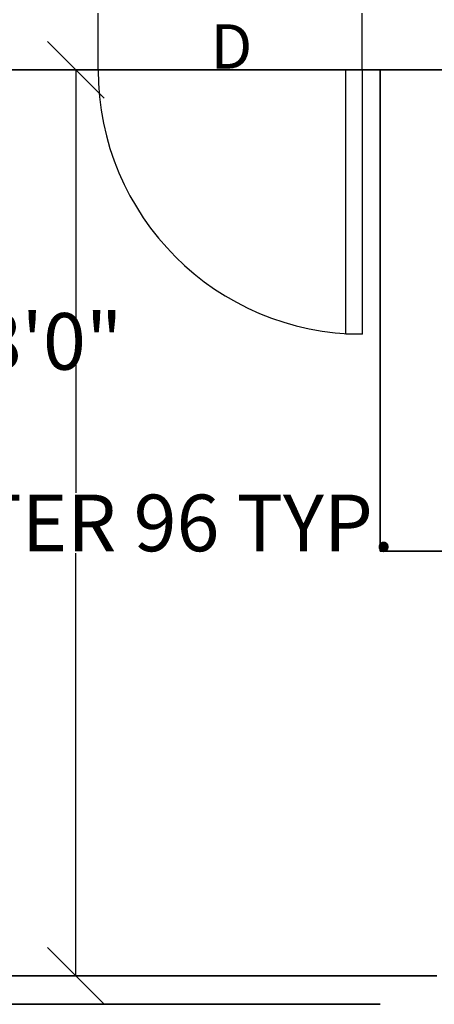
# Model space of a CAD drawing. Units: inches. Extents: x -1198 to -69, y -512 to 437.
# Tile 41 of 50: x -610 to -566, y 158 to 263. Entities that reach past the tile are written whole.
import ezdxf

# ---------------------------------------------------------------- set-up
doc = ezdxf.new("R2010")
doc.units = ezdxf.units.IN
doc.header["$MEASUREMENT"] = 0
for name, color, linetype, lineweight in [('A-ANNO-DIMS', 2, 'Continuous', 18), ('A-ANNO-SYMB', 7, 'Continuous', 18), ('A-AREA-IDEN', 7, 'Continuous', 18), ('A-WALL', 7, 'Continuous', 35), ('Doors', 140, 'Continuous', 25)]:
    doc.layers.add(name, color=color, linetype=linetype, lineweight=lineweight)
doc.styles.get("Standard").update_dxf_attribs({"font": 'arial.ttf'})
doc.dimstyles.get("Standard").update_dxf_attribs({"dimtxt": 6, "dimasz": 6, "dimexe": 0.18, "dimexo": 0.0625, "dimgap": 0.09, "dimtad": 0, "dimtih": 1, "dimtoh": 1, "dimdec": 0, "dimzin": 0, "dimdsep": 46, "dimlunit": 4, "dimtxsty": 'Standard', "dimblk": 'OBLIQUE', "dimcen": 0.09, "dimadec": 0, "dimazin": 0, "dimtfac": 1, "dimtdec": 0, "dimtofl": 0, "dimtmove": 0, "dimatfit": 3, "dimfxl": 1, "dimtolj": 1, "dimtzin": 0, "dimarcsym": 0})

# ---------------------------------------------------------------- blocks, each defined once
blk = doc.blocks.new('*U4')
for p, q in [((0, 0), (0, -6)), ((28, 0), (28, -6))]:
    blk.add_line(p, q)
blk.add_lwpolyline([(0, 0), (0, 28), (1.75, 28), (1.75, 0)], close=True)
blk.add_arc((0, 0), 28, 0, 90)
blk = doc.blocks.new('_Oblique')
at = {"color": 0, "linetype": 'ByBlock', "lineweight": -2}
blk.add_line((-0.5, -0.5), (0.5, 0.5), dxfattribs=at)
blk = doc.blocks.new('*D56')
at = {"layer": 'A-ANNO-DIMS', "color": 0, "lineweight": -2, "ltscale": 10, "transparency": 16777216}
for p, q in [((-618.34, 257.23), (-603.82, 257.23)), ((-604, 257.23), (-604, 212.42)), ((-604, 161.23), (-604, 206.03)), ((-618.34, 161.23), (-603.82, 161.23))]:
    blk.add_line(p, q, dxfattribs=at)
at = {"layer": 'DEFPOINTS', "color": 0, "ltscale": 10, "transparency": 16777216}
for p in [(-618.4, 257.23), (-604, 257.23), (-618.4, 161.23)]:
    blk.add_point(p, dxfattribs=at)
at = {"layer": 'A-ANNO-DIMS', "color": 0, "lineweight": -2, "ltscale": 10, "transparency": 16777216, "xscale": 6, "yscale": 6, "zscale": 6}
for p, rotation in [((-604, 257.23), 90), ((-604, 161.23), 270)]:
    blk.add_blockref('_Oblique', p, dxfattribs=dict(at, rotation=rotation))
at = {"layer": 'A-ANNO-DIMS', "color": 0, "ltscale": 10, "transparency": 16777216, "insert": (-604, 209.23), "char_height": 6, "attachment_point": 5}
blk.add_mtext('\\A1;COUNTER 96 TYP.', dxfattribs=at)

msp = doc.modelspace()

# ---------------------------------------------------------------- linework, layer by layer
at = {"layer": 'A-WALL', "ltscale": 10}
for p, q in [((-376.7509, 257.2277), (-691.7509, 257.2277)), ((-691.7509, 257.2277), (-601.6458, 257.2277)), ((-575.3958, 257.2277), (-571.7509, 257.2277)), ((-571.7509, 257.2277), (-571.7509, 206.2277)), ((-490.7509, 206.2277), (-571.7509, 206.2277)), ((-565.7509, 161.2277), (-691.7509, 161.2277)), ((-571.7509, 158.2277), (-691.7509, 158.2277))]:
    msp.add_line(p, q, dxfattribs=at)

# ---------------------------------------------------------------- block references
at = {"layer": 'Doors', "rotation": 180}
msp.add_blockref('*U4', (-573.6458, 257.2277), dxfattribs=at)

# ---------------------------------------------------------------- texts
at = {"layer": 'A-ANNO-SYMB', "ltscale": 10}
msp.add_text('D', height=4.6996, dxfattribs=at).set_placement((-589.7131, 257.3605))
at = {"layer": 'A-AREA-IDEN', "ltscale": 10, "insert": (-641.8292, 231.4637), "char_height": 6, "attachment_point": 1}
msp.add_mtext_dynamic_manual_height_columns('10\'0" x 8\'0"', width=57.976527, gutter_width=30, heights=[0], dxfattribs=at)

# ---------------------------------------------------------------- dimensions: what is measured, and where the dimension line sits
at = {"layer": 'A-ANNO-DIMS', "ltscale": 10}
dim = msp.add_linear_dim(base=(-604.0019, 257.2277), p1=(-618.4019, 161.2277), p2=(-618.4019, 257.2277), angle=90, text='COUNTER <> TYP.', dimstyle='Standard', override={"dimdec": 0, "dimlfac": 1, "dimrnd": 0, "dimzin": 0, "dimdsep": 46, "dimlunit": 2}, dxfattribs=at)
dim.commit()
dim.dimension.update_dxf_attribs({"geometry": '*D56', "text_midpoint": (-604.0019, 209.2277)})

doc.saveas('drawing.dxf')
